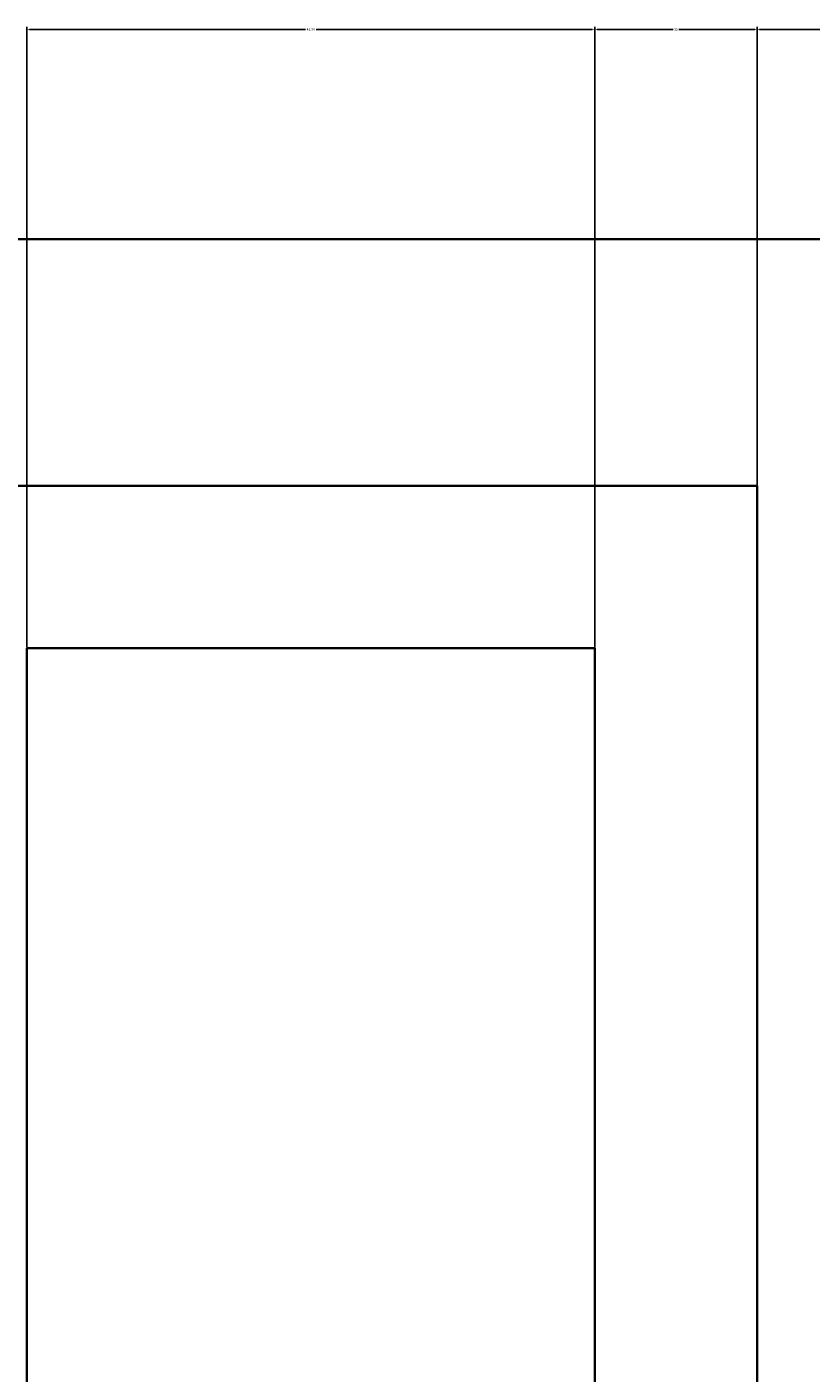
# Model space of a CAD drawing. Units: inches. Extents: x -6 to 289, y -8 to 323.
# Tile 47 of 107: x 46 to 104, y 223 to 323. Entities that reach past the tile are written whole.
import ezdxf

# ---------------------------------------------------------------- set-up
doc = ezdxf.new("R2010")
doc.units = ezdxf.units.IN
doc.header["$MEASUREMENT"] = 0
doc.layers.add('A-ANNO-DIMS', color=2, linetype='Continuous', lineweight=18)
doc.layers.add('A-ELEV', color=7, linetype='Continuous', lineweight=35)
doc.styles.get("Standard").update_dxf_attribs({"font": 'arial.ttf'})
doc.dimstyles.get("Standard").update_dxf_attribs({"dimtxt": 0.18, "dimasz": 0.18, "dimexe": 0.18, "dimexo": 0.0625, "dimgap": 0.09, "dimtad": 0, "dimtih": 1, "dimtoh": 1, "dimdec": 4, "dimzin": 0, "dimdsep": 46, "dimtxsty": 'Standard', "dimcen": 0.09, "dimadec": 0, "dimazin": 0, "dimtfac": 1, "dimtdec": 4, "dimtofl": 0, "dimtmove": 0, "dimatfit": 3, "dimfxl": 1, "dimtolj": 1, "dimtzin": 0, "dimarcsym": 0})

# ---------------------------------------------------------------- blocks, each defined once
blk = doc.blocks.new('*D7')
at = {"layer": 'A-ANNO-DIMS', "color": 0, "lineweight": -2, "transparency": 16777216}
for p, q in [((45.744, 277.105), (45.744, 322.969)), ((45.924, 322.789), (66.325, 322.789)), ((87.521, 322.789), (67.119, 322.789)), ((87.701, 277.105), (87.701, 322.969))]:
    blk.add_line(p, q, dxfattribs=at)
at = {"layer": 'A-ANNO-DIMS', "color": 0, "transparency": 16777216}
for points in [[(45.924, 322.819), (45.924, 322.759), (45.744, 322.789)], [(87.521, 322.819), (87.521, 322.759), (87.701, 322.789)]]:
    blk.add_solid(points, dxfattribs=at)
at = {"layer": 'Defpoints', "color": 0, "transparency": 16777216}
for p in [(87.701, 322.789), (45.744, 277.043), (87.701, 277.043)]:
    blk.add_point(p, dxfattribs=at)
at = {"layer": 'A-ANNO-DIMS', "color": 0, "transparency": 16777216, "insert": (66.722, 322.789), "char_height": 0.18, "attachment_point": 5}
blk.add_mtext('\\A1;41.96', dxfattribs=at)
blk = doc.blocks.new('*D8')
at = {"layer": 'A-ANNO-DIMS', "color": 0, "lineweight": -2, "transparency": 16777216}
for p, q in [((87.701, 277.105), (87.701, 322.969)), ((87.881, 322.789), (93.491, 322.789)), ((99.521, 322.789), (93.91, 322.789)), ((99.701, 289.105), (99.701, 322.969))]:
    blk.add_line(p, q, dxfattribs=at)
at = {"layer": 'A-ANNO-DIMS', "color": 0, "transparency": 16777216}
for points in [[(87.881, 322.819), (87.881, 322.759), (87.701, 322.789)], [(99.521, 322.819), (99.521, 322.759), (99.701, 322.789)]]:
    blk.add_solid(points, dxfattribs=at)
at = {"layer": 'Defpoints', "color": 0, "transparency": 16777216}
for p in [(99.701, 322.789), (99.701, 289.043), (87.701, 277.043)]:
    blk.add_point(p, dxfattribs=at)
at = {"layer": 'A-ANNO-DIMS', "color": 0, "transparency": 16777216, "insert": (93.701, 322.789), "char_height": 0.18, "attachment_point": 5}
blk.add_mtext('\\A1;12', dxfattribs=at)
blk = doc.blocks.new('*D9')
at = {"layer": 'A-ANNO-DIMS', "color": 0, "lineweight": -2, "transparency": 16777216}
for p, q in [((99.701, 289.105), (99.701, 322.969)), ((99.881, 322.789), (106.977, 322.789)), ((114.984, 322.789), (107.887, 322.789)), ((115.164, 307.351), (115.164, 322.969))]:
    blk.add_line(p, q, dxfattribs=at)
at = {"layer": 'A-ANNO-DIMS', "color": 0, "transparency": 16777216}
for points in [[(99.881, 322.819), (99.881, 322.759), (99.701, 322.789)], [(114.984, 322.819), (114.984, 322.759), (115.164, 322.789)]]:
    blk.add_solid(points, dxfattribs=at)
at = {"layer": 'Defpoints', "color": 0, "transparency": 16777216}
for p in [(115.164, 322.789), (115.164, 307.289), (99.701, 289.043)]:
    blk.add_point(p, dxfattribs=at)
at = {"layer": 'A-ANNO-DIMS', "color": 0, "transparency": 16777216, "insert": (107.432, 322.789), "char_height": 0.18, "attachment_point": 5}
blk.add_mtext('\\A1;15.463', dxfattribs=at)
blk = doc.blocks.new('*D27')
at = {"layer": 'A-ANNO-DIMS', "color": 0, "lineweight": -2, "transparency": 16777216}
for p, q in [((19.226, 307.289), (288.653, 307.289)), ((288.473, 307.109), (288.473, 277.471)), ((288.473, 247.469), (288.473, 277.107)), ((247.226, 247.289), (288.653, 247.289))]:
    blk.add_line(p, q, dxfattribs=at)
at = {"layer": 'A-ANNO-DIMS', "color": 0, "transparency": 16777216}
for points in [[(288.443, 307.109), (288.503, 307.109), (288.473, 307.289)], [(288.443, 247.469), (288.503, 247.469), (288.473, 247.289)]]:
    blk.add_solid(points, dxfattribs=at)
at = {"layer": 'Defpoints', "color": 0, "transparency": 16777216}
for p in [(19.164, 307.289), (288.473, 307.289), (247.164, 247.289)]:
    blk.add_point(p, dxfattribs=at)
at = {"layer": 'A-ANNO-DIMS', "color": 0, "transparency": 16777216, "insert": (288.473, 277.289), "char_height": 0.18, "attachment_point": 5}
blk.add_mtext('\\A1;60', dxfattribs=at)

msp = doc.modelspace()

# ---------------------------------------------------------------- linework, layer by layer
at = {"layer": 'A-ELEV'}
msp.add_line((118.1638, 307.2888), (19.1638, 307.2888), dxfattribs=at)
for points in [[(33.7437, 289.0427), (99.7007, 289.0427), (99.7007, 70.2425), (33.7437, 70.2425)], [(45.7437, 277.0427), (87.7007, 277.0427), (87.7007, 82.2425), (45.7437, 82.2425)]]:
    msp.add_lwpolyline(points, close=True, dxfattribs=at)

# ---------------------------------------------------------------- dimensions: what is measured, and where the dimension line sits
at = {"layer": 'A-ANNO-DIMS'}
for base, p1, p2, override, picture, middle in [((87.7007, 322.7888), (45.7437, 277.0427), (87.7007, 277.0427), {"dimdec": 2, "dimlfac": 1, "dimrnd": 0, "dimzin": 0, "dimdsep": 46, "dimlunit": 2}, '*D7', (66.7222, 322.7888)), ((99.7007, 322.7888), (87.7007, 277.0427), (99.7007, 289.0427), {"dimdec": 0, "dimlfac": 1, "dimrnd": 0, "dimzin": 0, "dimdsep": 46, "dimlunit": 2}, '*D8', (93.7007, 322.7888)), ((115.1638, 322.7888), (99.7007, 289.0427), (115.1638, 307.2888), {"dimdec": 3, "dimlfac": 1, "dimrnd": 0, "dimzin": 0, "dimdsep": 46, "dimlunit": 2}, '*D9', (107.4322, 322.7888))]:
    dim = msp.add_linear_dim(base=base, p1=p1, p2=p2, dimstyle='Standard', override=override, dxfattribs=at)
    dim.commit()
    dim.dimension.update_dxf_attribs({"geometry": picture, "text_midpoint": middle})
dim = msp.add_linear_dim(base=(288.4733, 307.2888), p1=(247.1638, 247.2888), p2=(19.1638, 307.2888), angle=90, dimstyle='Standard', override={"dimdec": 0, "dimlfac": 1, "dimrnd": 0, "dimzin": 0, "dimdsep": 46, "dimlunit": 2}, dxfattribs=at)
dim.commit()
dim.dimension.update_dxf_attribs({"geometry": '*D27', "text_midpoint": (288.4733, 277.2888)})

doc.saveas('drawing.dxf')
